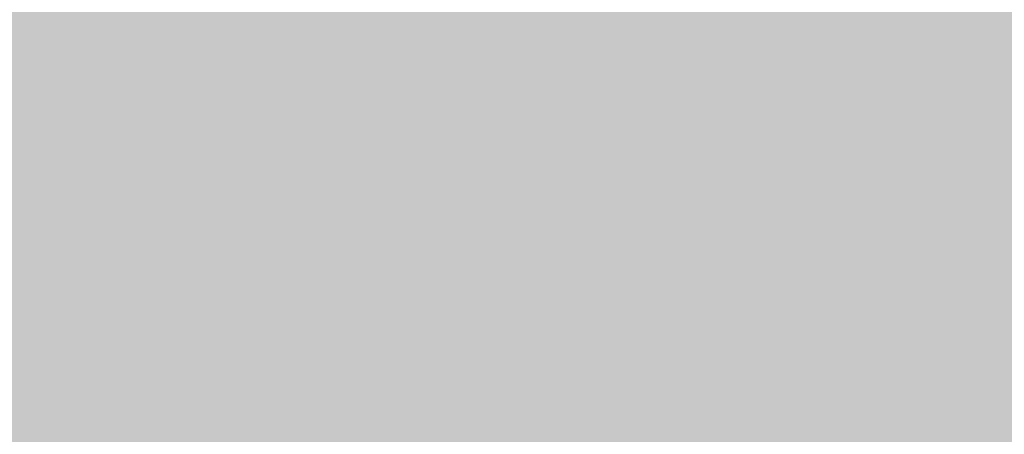
# Model space of a CAD drawing. Units: feet. Extents: x 3168 to 4724, y 827 to 1477.
# Tile 68 of 256: x 3273.17306 to 3273.20669, y 1099.00068 to 1099.01485. Entities that reach past the tile are written whole.
import ezdxf

# ---------------------------------------------------------------- set-up
doc = ezdxf.new("R2010")
doc.units = ezdxf.units.FT
doc.layers.add('A-ELEV', color=7, linetype='Continuous', lineweight=35)
doc.layers.add('A-ELEV-PATT', color=8, linetype='Continuous', lineweight=13)

msp = doc.modelspace()

# ---------------------------------------------------------------- hatches: boundary and pattern name
at = {"layer": 'A-ELEV-PATT'}
h = msp.add_hatch(color=256, dxfattribs=at)
h.dxf.hatch_style = 1
edge = h.paths.add_edge_path()
edge.add_ellipse((3552.905762, 979.220141), major_axis=(36.744924, 0), ratio=0.484848485, start_angle=0, end_angle=360)
edge = h.paths.add_edge_path()
edge.add_ellipse((3559.891637, 929.252282), major_axis=(36.744924, 0), ratio=0.484848485, start_angle=0, end_angle=360)
edge = h.paths.add_edge_path()
edge.add_line((3299.31681, 1198.606081), (3479.916714, 1198.606081))
edge.add_line((3479.916714, 1198.606081), (3479.916714, 1209.86857))
edge.add_spline(control_points=[(3479.916714, 1209.86857), (3464.301157, 1209.86857), (3448.685601, 1209.86857), (3410.949139, 1209.86857), (3388.828234, 1209.86857), (3355.646876, 1209.86857), (3344.586423, 1209.86857), (3327.995745, 1209.86857), (3322.465518, 1209.86857), (3314.170179, 1209.86857), (3311.405066, 1209.86857), (3307.257396, 1209.86857), (3305.874839, 1209.86857), (3303.801005, 1209.86857), (3303.109726, 1209.86857), (3302.072809, 1209.86857), (3301.72717, 1209.86857), (3301.208711, 1209.86857), (3301.035891, 1209.86857), (3300.776662, 1209.86857), (3300.690252, 1209.86857), (3300.560638, 1209.86857), (3300.517433, 1209.86857), (3300.452625, 1209.86857), (3300.431023, 1209.86857), (3300.398619, 1209.86857), (3300.387818, 1209.86857), (3300.366216, 1209.86857), (3300.345676, 1209.86857), (3300.345548, 1209.86857), (3300.345505, 1209.86857), (3300.343304, 1209.86857), (3300.341146, 1209.868571), (3300.337909, 1209.868571), (3300.33683, 1209.868572), (3300.333942, 1209.868573), (3300.332133, 1209.868574), (3300.325515, 1209.868577), (3300.320706, 1209.868581), (3300.310925, 1209.868592), (3300.305952, 1209.868598), (3300.290511, 1209.868623), (3300.280045, 1209.868646), (3300.232425, 1209.868777), (3300.195298, 1209.868954), (3299.951068, 1209.870608), (3299.744824, 1209.874326), (3299.436827, 1209.883257), (3299.334389, 1209.886792), (3299.181079, 1209.89292), (3299.130033, 1209.895099), (3298.652217, 1209.916801), (3298.22946, 1209.945718), (3297.601631, 1210.002367), (3297.393404, 1210.023464), (3297.082652, 1210.058309), (3296.979332, 1210.070458), (3296.292954, 1210.154861), (3295.718148, 1210.243356), (3294.868717, 1210.39885), (3294.5877, 1210.454478), (3294.169341, 1210.543349), (3294.030415, 1210.573878), (3291.707149, 1211.1012), (3289.65359, 1211.813435), (3285.776259, 1213.563988), (3283.95141, 1214.603478), (3280.512159, 1216.98008), (3278.897241, 1218.317592), (3276.379914, 1220.829489), (3275.416042, 1221.917738), (3274.039342, 1223.7077), (3273.581043, 1224.349535), (3273.143228, 1225.016316)], knot_values=[39.119033, 39.119033, 39.119033, 39.119033, 39.286353, 39.286353, 39.523379, 39.523379, 39.641892, 39.641892, 39.701148, 39.701148, 39.730777, 39.730777, 39.745591, 39.745591, 39.752998, 39.752998, 39.756701, 39.756701, 39.758553, 39.758553, 39.759479, 39.759479, 39.759942, 39.759942, 39.760173, 39.760173, 39.760289, 39.760289, 39.760405, 39.760405, 39.760463, 39.760463, 39.763389, 39.763389, 39.764851, 39.764851, 39.767304, 39.767304, 39.773825, 39.773825, 39.78057, 39.78057, 39.79477, 39.79477, 39.845194, 39.845194, 40.126715, 40.126715, 40.267476, 40.267476, 40.337856, 40.337856, 40.927023, 40.927023, 41.221606, 41.221606, 41.368898, 41.368898, 42.202622, 42.202622, 42.619485, 42.619485, 42.827916, 42.827916, 46.118323, 46.118323, 49.408731, 49.408731, 52.699139, 52.699139, 54.927489, 54.927489, 56.104228, 56.104228, 56.104228, 56.104228], weights=[1, 1, 1, 1, 1, 1, 1, 1, 1, 1, 1, 1, 1, 1, 1, 1, 1, 1, 1, 1, 1, 1, 1, 1, 1, 1, 1, 1, 1, 1, 1, 1, 1, 1, 1, 1, 1, 1, 1, 1, 1, 1, 1, 1, 1, 1, 1, 1, 1, 1, 1, 1, 1, 1, 1, 1, 1, 1, 1, 1, 1, 1, 1, 1, 1, 1, 1, 1, 1, 1, 1, 1, 1, 1], degree=3, periodic=0)
edge.add_line((3273.143228, 1225.016316), (3273.143228, 1099.016316))
edge.add_line((3273.143228, 1099.016316), (3299.31681, 1099.016316))
edge.add_line((3299.31681, 1099.016316), (3299.31681, 1198.606081))
edge = h.paths.add_edge_path()
edge.add_line((3304.758443, 1324.15806), (3479.916714, 1324.15806))
edge.add_line((3479.916714, 1324.15806), (3479.916714, 1335.714618))
edge.add_line((3479.916714, 1335.714618), (3269.161628, 1335.714618))
edge.add_spline(control_points=[(3269.161628, 1335.714618), (3264.024231, 1335.714618), (3258.364118, 1328.958189), (3259.264311, 1323.900274)], knot_values=[0, 0, 0, 0, 15.412191, 15.412191, 15.412191, 15.412191], degree=3, periodic=0)
edge.add_line((3259.264311, 1323.900274), (3265.516849, 1288.769135))
edge.add_line((3265.516849, 1288.769135), (3275.265103, 1261.545626))
edge.add_line((3275.265103, 1261.545626), (3304.758443, 1261.545626))
edge.add_line((3304.758443, 1261.545626), (3304.758443, 1324.15806))
h = msp.add_hatch(color=256, dxfattribs=at)
h.dxf.hatch_style = 1
h.paths.add_polyline_path([(3384.525247, 1099.016316), (3335.029168, 1099.016316), (3299.31681, 1099.016316), (3273.143228, 1099.016316), (3217.565364, 1099.016316), (3168.069285, 827.11626), (3335.029168, 827.11626)])

# ---------------------------------------------------------------- linework, layer by layer
at = {"layer": 'A-ELEV'}
msp.add_open_spline([(3808.5202, 1099.016316), (3808.5202, 1141.413235), (3808.5202, 1183.810154), (3808.5202, 1226.635324), (3808.5202, 1227.063576), (3808.5202, 1227.491828), (3811.491871, 1248.994673), (3814.463542, 1270.497518), (3817.46523, 1292.217564), (3817.495247, 1292.434764), (3817.525264, 1292.651964), (3817.572801, 1310.106748), (3817.620339, 1327.561532), (3817.667877, 1345.016316), (3817.667877, 1345.457962), (3817.667877, 1345.899608), (3817.667877, 1346.456047), (3817.667877, 1346.57084), (3817.667877, 1346.752887), (3817.667877, 1346.820142), (3817.667877, 1346.93487), (3817.667877, 1346.982345), (3817.667877, 1347.038587), (3817.667877, 1347.047356), (3817.667877, 1347.073661), (3817.667877, 1347.059303), (3817.667877, 1347.061545), (3817.667876, 1347.062667), (3817.667875, 1347.066031), (3817.667874, 1347.068274), (3817.66787, 1347.075001), (3817.667866, 1347.079486), (3817.667849, 1347.092937), (3817.667833, 1347.101902), (3817.667766, 1347.12879), (3817.667699, 1347.146705), (3817.667432, 1347.200421), (3817.667165, 1347.236192), (3817.6661, 1347.343385), (3817.665038, 1347.414686), (3817.660812, 1347.628095), (3817.656608, 1347.769708), (3817.63997, 1348.192487), (3817.623509, 1348.471586), (3817.559094, 1349.300067), (3817.496121, 1349.840588), (3817.255432, 1351.424156), (3817.026318, 1352.428785), (3816.306871, 1354.888914), (3815.743745, 1356.268727), (3814.463959, 1358.81921), (3813.746413, 1359.990968), (3812.195838, 1362.172343), (3811.362245, 1363.182124), (3809.588836, 1365.069009), (3808.648816, 1365.946105), (3806.654262, 1367.579616), (3805.599702, 1368.336154), (3803.352891, 1369.722327), (3802.160535, 1370.352386), (3799.600813, 1371.453586), (3798.232688, 1371.925481), (3795.280084, 1372.634624), (3793.693148, 1372.872068), (3791.869441, 1372.92648), (3791.740861, 1372.92922), (3791.353371, 1372.934101), (3791.092707, 1372.932901), (3790.304116, 1372.915068), (3789.769543, 1372.884195), (3789.20919, 1372.830236), (3789.190622, 1372.828424), (3789.134892, 1372.822912), (3789.097705, 1372.819137), (3789.048445, 1372.814008), (3789.0364, 1372.812743), (3789.000256, 1372.808918), (3788.976147, 1372.806325), (3788.949405, 1372.803404), (3788.946786, 1372.803118), (3788.942567, 1372.802655), (3788.940967, 1372.80248), (3788.938572, 1372.802217), (3788.937777, 1372.802129), (3788.935391, 1372.801867), (3788.867535, 1372.794402), (3788.756866, 1372.782228), (3788.701532, 1372.776141), (3788.53553, 1372.75788), (3788.424861, 1372.745707), (3788.092856, 1372.709185), (3787.871519, 1372.684837), (3787.207509, 1372.611793), (3786.764835, 1372.563097), (3785.436814, 1372.417009), (3784.551467, 1372.319617), (3781.895425, 1372.027442), (3780.12473, 1371.832658), (3774.812646, 1371.248307), (3771.271256, 1370.858739), (3760.647088, 1369.690037), (3753.56431, 1368.910902), (3732.315973, 1366.573498), (3718.150416, 1365.015228), (3694.006758, 1362.359326), (3684.028657, 1361.261694), (3674.050557, 1360.164062), (3664.600662, 1360.164062), (3655.150767, 1360.164062), (3626.801081, 1360.164062), (3607.901291, 1360.164062), (3551.20192, 1360.164062), (3513.40234, 1360.164062), (3467.725182, 1360.164062), (3459.847604, 1360.164062), (3436.214873, 1360.164062), (3420.459718, 1360.164062), (3373.194255, 1360.164062), (3341.683946, 1360.164062), (3302.848162, 1360.164062), (3295.522686, 1360.164062), (3286.038292, 1360.164062), (3283.879372, 1360.164062), (3277.402613, 1360.164062), (3273.084773, 1360.164062), (3267.732851, 1360.164062), (3266.698768, 1360.164062), (3263.59652, 1360.164062), (3261.528355, 1360.164062), (3259.236943, 1360.164062), (3259.013697, 1360.164062), (3258.343958, 1360.164062), (3257.897466, 1360.164062), (3257.430998, 1360.164062), (3257.411022, 1360.164062), (3257.370573, 1360.164062), (3257.37547, 1360.164062), (3257.374598, 1360.164062), (3257.373937, 1360.164062), (3257.371956, 1360.164062), (3257.370635, 1360.164061), (3257.366673, 1360.16406), (3257.364032, 1360.164059), (3257.356109, 1360.164053), (3257.350828, 1360.164047), (3257.334987, 1360.164023), (3257.32443, 1360.163998), (3257.292769, 1360.163899), (3257.271676, 1360.163799), (3257.208439, 1360.163398), (3257.166337, 1360.162995), (3257.040206, 1360.161388), (3256.956349, 1360.159783), (3256.705504, 1360.153393), (3256.53924, 1360.147036), (3256.04357, 1360.121916), (3255.717296, 1360.097102), (3254.752446, 1360.000481), (3254.127968, 1359.906513), (3252.180067, 1359.525332), (3250.941574, 1359.143991), (3248.670175, 1358.24329), (3247.635739, 1357.723834), (3245.732632, 1356.603471), (3244.863388, 1356.00206), (3243.253108, 1354.742865), (3242.511972, 1354.084731), (3240.751052, 1352.344781), (3239.800961, 1351.229574), (3238.087769, 1348.87244), (3237.324685, 1347.630355), (3235.98251, 1344.971632), (3235.402205, 1343.554907), (3234.591081, 1340.815458), (3234.310882, 1339.54355), (3233.97649, 1336.802561), (3233.922113, 1335.330877), (3234.148916, 1332.591269), (3234.349529, 1331.367201), (3234.719893, 1329.999367), (3234.752423, 1329.883362), (3234.853619, 1329.534797), (3234.925892, 1329.301685), (3235.024836, 1329.002552), (3235.046924, 1328.936928), (3235.077639, 1328.847239), (3235.085924, 1328.823198), (3235.110939, 1328.751064), (3235.127828, 1328.702962), (3235.147992, 1328.646242), (3235.151059, 1328.637632), (3235.156096, 1328.623526), (3235.158061, 1328.61803), (3235.160209, 1328.61203), (3235.165612, 1328.596943), (3235.180099, 1328.556486), (3235.190263, 1328.528101), (3235.220756, 1328.442946), (3235.241084, 1328.386176), (3235.302069, 1328.215865), (3235.342726, 1328.102325), (3235.464696, 1327.761704), (3235.54601, 1327.534623), (3235.78995, 1326.853381), (3235.952577, 1326.39922), (3236.440459, 1325.036736), (3236.765713, 1324.128414), (3237.741475, 1321.403446), (3238.391983, 1319.586801), (3240.343508, 1314.136866), (3241.644525, 1310.503576), (3245.547574, 1299.603706), (3248.149607, 1292.337126), (3255.955706, 1270.537385), (3261.159772, 1256.004225), (3267.387618, 1238.612001), (3268.411397, 1235.752937), (3269.510378, 1232.683864), (3269.585579, 1232.473854), (3269.706612, 1232.135851), (3269.752444, 1232.007857), (3269.827329, 1231.79873), (3269.856382, 1231.717595), (3269.906325, 1231.578122), (3269.927215, 1231.519782), (3269.972468, 1231.393406), (3269.996831, 1231.325368), (3270.026503, 1231.242506), (3270.031811, 1231.227681), (3270.040282, 1231.204024), (3270.039224, 1231.206979), (3270.039359, 1231.206601), (3270.039427, 1231.206412), (3270.03963, 1231.205846), (3270.039765, 1231.205468), (3270.040171, 1231.204335), (3270.040442, 1231.203579), (3270.041254, 1231.201313), (3270.041796, 1231.199802), (3270.04342, 1231.195269), (3270.044504, 1231.192248), (3270.047756, 1231.183185), (3270.049926, 1231.177145), (3270.056442, 1231.159028), (3270.060793, 1231.146957), (3270.073867, 1231.110761), (3270.082613, 1231.086656), (3270.108936, 1231.014413), (3270.1266, 1230.96635), (3270.179934, 1230.822457), (3270.215947, 1230.726923), (3270.325323, 1230.441508), (3270.400026, 1230.252811), (3270.629249, 1229.691444), (3270.788883, 1229.323501), (3271.286488, 1228.238319), (3271.6431, 1227.539755), (3272.775859, 1225.515277), (3273.614169, 1224.260502), (3275.416042, 1221.917738), (3276.379914, 1220.829489), (3278.897241, 1218.317592), (3280.512159, 1216.98008), (3283.95141, 1214.603478), (3285.776259, 1213.563988), (3289.65359, 1211.813435), (3291.707149, 1211.1012), (3294.030415, 1210.573878), (3294.169341, 1210.543349), (3294.5877, 1210.454478), (3294.868717, 1210.39885), (3295.718148, 1210.243356), (3296.292954, 1210.154861), (3296.979332, 1210.070458), (3297.082652, 1210.058309), (3297.393404, 1210.023464), (3297.601631, 1210.002367), (3298.22946, 1209.945718), (3298.652217, 1209.916801), (3299.130033, 1209.895099), (3299.181079, 1209.89292), (3299.334389, 1209.886792), (3299.436827, 1209.883257), (3299.744824, 1209.874326), (3299.951068, 1209.870608), (3300.195298, 1209.868954), (3300.232425, 1209.868777), (3300.280045, 1209.868646), (3300.290511, 1209.868623), (3300.305952, 1209.868598), (3300.310925, 1209.868592), (3300.320706, 1209.868581), (3300.325515, 1209.868577), (3300.332133, 1209.868574), (3300.333942, 1209.868573), (3300.33683, 1209.868572), (3300.337909, 1209.868571), (3300.341146, 1209.868571), (3300.343304, 1209.86857), (3300.345505, 1209.86857), (3300.345548, 1209.86857), (3300.345676, 1209.86857), (3300.366216, 1209.86857), (3300.387818, 1209.86857), (3300.398619, 1209.86857), (3300.431023, 1209.86857), (3300.452625, 1209.86857), (3300.517433, 1209.86857), (3300.560638, 1209.86857), (3300.690252, 1209.86857), (3300.776662, 1209.86857), (3301.035891, 1209.86857), (3301.208711, 1209.86857), (3301.72717, 1209.86857), (3302.072809, 1209.86857), (3303.109726, 1209.86857), (3303.801005, 1209.86857), (3305.874839, 1209.86857), (3307.257396, 1209.86857), (3311.405066, 1209.86857), (3314.170179, 1209.86857), (3322.465518, 1209.86857), (3327.995745, 1209.86857), (3344.586423, 1209.86857), (3355.646876, 1209.86857), (3388.828234, 1209.86857), (3410.949139, 1209.86857), (3477.311855, 1209.86857), (3521.553665, 1209.86857), (3566.836184, 1209.86857), (3567.876892, 1209.86857), (3570.999017, 1209.86857), (3573.080433, 1209.86857), (3575.781396, 1209.86857), (3576.400943, 1209.86857), (3577.295821, 1209.86857), (3577.571152, 1209.86857), (3578.397146, 1209.86857), (3578.947808, 1209.86857), (3579.756491, 1209.86857), (3580.014511, 1209.86857), (3580.342737, 1209.86857), (3580.326865, 1209.86857), (3580.32717, 1209.86857), (3580.327323, 1209.86857), (3580.327781, 1209.86857), (3580.328086, 1209.86857), (3580.329002, 1209.86857), (3580.329613, 1209.86857), (3580.331445, 1209.86857), (3580.332667, 1209.86857), (3580.336332, 1209.868569), (3580.338775, 1209.868567), (3580.346107, 1209.868563), (3580.350995, 1209.868558), (3580.365663, 1209.86854), (3580.375445, 1209.868522), (3580.404801, 1209.868449), (3580.424386, 1209.868376), (3580.483183, 1209.868085), (3580.522437, 1209.867793), (3580.640361, 1209.866624), (3580.719195, 1209.865454), (3580.956315, 1209.860766), (3581.115222, 1209.85607), (3581.594164, 1209.83723), (3581.916419, 1209.818331), (3582.889947, 1209.742428), (3583.547986, 1209.666169), (3585.531827, 1209.360617), (3586.867216, 1209.053886), (3589.471545, 1208.252472), (3590.740241, 1207.757852), (3591.995451, 1207.158802), (3592.057809, 1207.12874), (3592.244242, 1207.037954), (3592.367676, 1206.976632), (3592.73528, 1206.790359), (3592.976752, 1206.663101), (3593.244539, 1206.516441), (3593.274731, 1206.499825), (3593.365115, 1206.449839), (3593.425113, 1206.416333), (3593.604314, 1206.315285), (3593.722725, 1206.247211), (3593.857212, 1206.168398), (3593.874362, 1206.158319), (3593.925741, 1206.128041), (3593.959899, 1206.107798), (3594.062086, 1206.046899), (3594.129827, 1206.006074), (3594.208436, 1205.958171), (3594.219683, 1205.951304), (3594.253391, 1205.930686), (3594.275819, 1205.916917), (3594.342972, 1205.875536), (3594.387563, 1205.847853), (3594.433616, 1205.81905), (3594.435256, 1205.818024), (3594.440175, 1205.814946), (3594.443453, 1205.812894), (3594.447123, 1205.810594), (3594.447516, 1205.810348), (3594.448695, 1205.80961), (3594.449481, 1205.809117), (3594.450366, 1205.808562), (3594.450466, 1205.8085), (3594.4506, 1205.808415), (3594.467399, 1205.797887), (3594.493269, 1205.781674), (3594.506204, 1205.773568), (3594.545008, 1205.749248), (3594.570878, 1205.733035), (3594.648487, 1205.684396), (3594.700226, 1205.651969), (3594.855444, 1205.554691), (3594.958922, 1205.489839), (3595.269357, 1205.295282), (3595.476314, 1205.165577), (3596.097185, 1204.776463), (3596.511099, 1204.517054), (3597.752841, 1203.738826), (3598.580669, 1203.220007), (3601.064152, 1201.663551), (3602.719807, 1200.625914), (3607.686774, 1197.513002), (3610.998085, 1195.437727), (3620.932018, 1189.211903), (3627.55464, 1185.061354), (3647.422507, 1172.609707), (3660.667751, 1164.308608), (3700.403484, 1139.405313), (3726.893973, 1122.803116), (3757.205715, 1103.806052), (3761.02697, 1101.411184), (3764.848224, 1099.016316), (3745.328271, 1099.016316), (3725.808319, 1099.016316), (3706.288366, 1099.016316), (3706.288366, 1108.453237), (3706.288366, 1117.890158), (3706.288366, 1127.327079), (3710.750754, 1127.327079), (3715.213143, 1127.327079), (3719.675531, 1127.327079)], degree=3, knots=[0, 0, 0, 0, 0.982037, 0.982037, 0.991957, 0.991957, 0.991957, 1.966522, 1.966522, 1.976367, 1.976367, 1.976367, 2.976367, 2.976367, 2.976367, 3.00169, 3.00169, 3.008272, 3.008272, 3.012129, 3.012129, 3.014851, 3.014851, 3.015353, 3.015353, 3.016359, 3.016359, 3.017365, 3.017365, 3.019376, 3.019376, 3.023398, 3.023398, 3.031442, 3.031442, 3.047531, 3.047531, 3.079708, 3.079708, 3.144063, 3.144063, 3.272772, 3.272772, 3.53019, 3.53019, 4.045026, 4.045026, 5.074698, 5.074698, 6.700878, 6.700878, 8.327058, 8.327058, 9.953238, 9.953238, 11.579418, 11.579418, 13.205598, 13.205598, 14.831778, 14.831778, 16.457958, 16.457958, 18.084138, 18.084138, 18.206872, 18.206872, 18.45234, 18.45234, 18.943275, 18.943275, 18.960093, 18.960093, 18.993729, 18.993729, 19.00461, 19.00461, 19.026374, 19.026374, 19.028737, 19.028737, 19.03018, 19.03018, 19.030897, 19.030897, 19.032332, 19.032332, 19.033766, 19.033766, 19.036636, 19.036636, 19.042374, 19.042374, 19.053851, 19.053851, 19.076805, 19.076805, 19.122714, 19.122714, 19.21453, 19.21453, 19.398163, 19.398163, 19.765429, 19.765429, 20.024128, 20.024128, 20.024128, 20.092031, 20.092031, 20.227836, 20.227836, 20.499446, 20.499446, 20.556051, 20.556051, 20.66926, 20.66926, 20.895678, 20.895678, 20.948316, 20.948316, 20.963829, 20.963829, 20.994855, 20.994855, 21.002285, 21.002285, 21.017146, 21.017146, 21.01875, 21.01875, 21.021959, 21.021959, 21.022102, 21.022102, 21.022249, 21.022249, 21.022708, 21.022708, 21.023627, 21.023627, 21.025464, 21.025464, 21.029138, 21.029138, 21.036486, 21.036486, 21.051183, 21.051183, 21.080575, 21.080575, 21.139361, 21.139361, 21.256932, 21.256932, 21.492073, 21.492073, 21.962356, 21.962356, 23.01002, 23.01002, 24.057684, 24.057684, 25.105348, 25.105348, 26.153011, 26.153011, 27.776787, 27.776787, 29.400562, 29.400562, 31.024337, 31.024337, 32.278801, 32.278801, 33.533265, 33.533265, 34.467568, 34.467568, 34.553971, 34.553971, 34.726776, 34.726776, 34.775309, 34.775309, 34.793079, 34.793079, 34.82862, 34.82862, 34.834979, 34.834979, 34.839039, 34.839039, 34.839411, 34.839411, 34.840285, 34.840285, 34.842034, 34.842034, 34.845531, 34.845531, 34.852525, 34.852525, 34.866512, 34.866512, 34.894488, 34.894488, 34.950439, 34.950439, 35.062342, 35.062342, 35.286147, 35.286147, 35.733758, 35.733758, 35.821815, 35.821815, 35.828283, 35.828283, 35.832225, 35.832225, 35.834724, 35.834724, 35.836521, 35.836521, 35.838617, 35.838617, 35.839073, 35.839073, 35.839345, 35.839345, 35.839617, 35.839617, 35.840161, 35.840161, 35.841249, 35.841249, 35.843425, 35.843425, 35.847778, 35.847778, 35.856482, 35.856482, 35.873891, 35.873891, 35.908709, 35.908709, 35.978345, 35.978345, 36.117617, 36.117617, 36.396161, 36.396161, 36.953248, 36.953248, 38.067423, 38.067423, 40.295772, 40.295772, 42.524122, 42.524122, 45.81453, 45.81453, 49.104937, 49.104937, 52.395345, 52.395345, 52.603776, 52.603776, 53.020639, 53.020639, 53.854363, 53.854363, 54.001655, 54.001655, 54.296238, 54.296238, 54.885405, 54.885405, 54.955785, 54.955785, 55.096546, 55.096546, 55.378067, 55.378067, 55.42849, 55.42849, 55.442691, 55.442691, 55.449436, 55.449436, 55.455957, 55.455957, 55.458409, 55.458409, 55.459872, 55.459872, 55.462798, 55.462798, 55.462856, 55.462856, 55.462972, 55.462972, 55.463088, 55.463088, 55.463319, 55.463319, 55.463782, 55.463782, 55.464708, 55.464708, 55.46656, 55.46656, 55.470263, 55.470263, 55.47767, 55.47767, 55.492484, 55.492484, 55.522112, 55.522112, 55.581369, 55.581369, 55.699882, 55.699882, 55.936907, 55.936907, 56.410959, 56.410959, 56.42211, 56.42211, 56.444413, 56.444413, 56.451051, 56.451051, 56.454001, 56.454001, 56.459901, 56.459901, 56.462666, 56.462666, 56.463418, 56.463418, 56.464171, 56.464171, 56.465675, 56.465675, 56.468684, 56.468684, 56.474702, 56.474702, 56.486738, 56.486738, 56.51081, 56.51081, 56.558955, 56.558955, 56.655243, 56.655243, 56.847821, 56.847821, 57.232975, 57.232975, 58.003284, 58.003284, 59.543901, 59.543901, 62.625137, 62.625137, 68.787607, 68.787607, 74.950078, 74.950078, 75.27336, 75.27336, 75.919923, 75.919923, 77.213051, 77.213051, 77.377769, 77.377769, 77.707206, 77.707206, 78.366079, 78.366079, 78.462532, 78.462532, 78.655436, 78.655436, 79.041245, 79.041245, 79.105735, 79.105735, 79.234714, 79.234714, 79.492672, 79.492672, 79.502197, 79.502197, 79.521249, 79.521249, 79.523534, 79.523534, 79.528103, 79.528103, 79.528682, 79.528682, 79.528885, 79.528885, 79.529089, 79.529089, 79.529495, 79.529495, 79.530308, 79.530308, 79.531935, 79.531935, 79.535187, 79.535187, 79.541693, 79.541693, 79.554704, 79.554704, 79.580725, 79.580725, 79.632769, 79.632769, 79.736856, 79.736856, 79.94503, 79.94503, 80.361377, 80.361377, 80.421435, 80.421435, 80.421435, 81.421435, 81.421435, 81.421435, 82.421435, 82.421435, 82.421435, 83.421435, 83.421435, 83.421435, 83.421435], dxfattribs=at)

doc.saveas('drawing.dxf')
